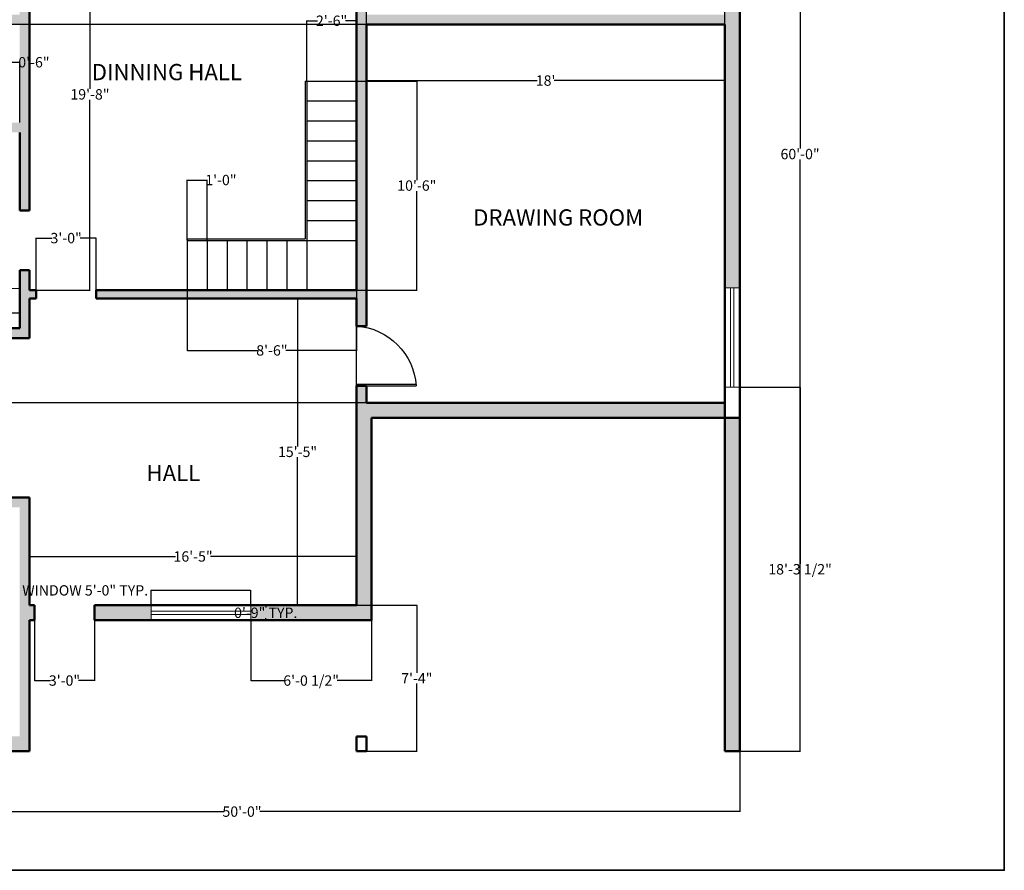
# Model space of a CAD drawing. Units: inches. Extents: x -335 to 1312, y -66 to 821.
# Tile 3 of 4: x 719 to 1312, y -66 to 446. Entities that reach past the tile are written whole.
import ezdxf

# ---------------------------------------------------------------- set-up
doc = ezdxf.new("R2010")
doc.units = ezdxf.units.IN
doc.header["$MEASUREMENT"] = 0
for name, color, linetype, lineweight in [('A-ANNO-DIMS', 2, 'Continuous', 18), ('A-ANNO-TTLB', 7, 'Continuous', 35), ('A-AREA-IDEN', 7, 'Continuous', 25), ('A-COLS', 7, 'Continuous', 50), ('A-DOOR', 34, 'Continuous', 25), ('A-FLOR-FIXT', 8, 'Continuous', 18), ('A-FLOR-STRS', 7, 'Continuous', 25), ('A-GLAZ', 34, 'Continuous', 18), ('A-WALL', 7, 'Continuous', 50), ('A-WALL-PATT', 252, 'Continuous', 13)]:
    doc.layers.add(name, color=color, linetype=linetype, lineweight=lineweight)
doc.styles.get("Standard").update_dxf_attribs({"font": 'arial.ttf'})
doc.dimstyles.get("Standard").update_dxf_attribs({"dimtxt": 6.25, "dimasz": 0.18, "dimexe": 0.18, "dimexo": 0.0625, "dimgap": 0.09, "dimtad": 0, "dimtih": 1, "dimtoh": 1, "dimdec": 0, "dimzin": 0, "dimdsep": 46, "dimlunit": 3, "dimtxsty": 'Standard', "dimcen": 0.09, "dimadec": 0, "dimazin": 0, "dimtfac": 1, "dimtdec": 0, "dimtofl": 0, "dimtmove": 0, "dimatfit": 3, "dimfxl": 1, "dimtolj": 1, "dimtzin": 0, "dimarcsym": 0})

# ---------------------------------------------------------------- blocks, each defined once
blk = doc.blocks.new('*D6')
at = {"layer": 'A-ANNO-DIMS', "color": 0, "lineweight": -2, "transparency": 16777216}
for p, q in [((561.55, 260.47), (561.55, 269.75)), ((561.73, 269.57), (629.52, 269.57)), ((718.37, 269.57), (650.58, 269.57)), ((718.55, 260.47), (718.55, 269.75))]:
    blk.add_line(p, q, dxfattribs=at)
at = {"layer": 'A-ANNO-DIMS', "color": 0, "transparency": 16777216}
for points in [[(561.73, 269.6), (561.73, 269.54), (561.55, 269.57)], [(718.37, 269.6), (718.37, 269.54), (718.55, 269.57)]]:
    blk.add_solid(points, dxfattribs=at)
at = {"layer": 'Defpoints', "color": 0, "transparency": 16777216}
for p in [(561.55, 269.57), (561.55, 260.41), (718.55, 260.41)]:
    blk.add_point(p, dxfattribs=at)
at = {"layer": 'A-ANNO-DIMS', "color": 0, "transparency": 16777216, "insert": (640.05, 269.57), "char_height": 6.25, "attachment_point": 5}
blk.add_mtext('\\A1;13\'-1"', dxfattribs=at)
blk = doc.blocks.new('*D15')
at = {"layer": 'A-ANNO-DIMS', "color": 0, "lineweight": -2, "transparency": 16777216}
for p, q in [((921.49, 278.41), (885.84, 278.41)), ((886.02, 278.23), (886.02, 189.19)), ((886.02, 93.59), (886.02, 182.63)), ((921.49, 93.41), (885.84, 93.41))]:
    blk.add_line(p, q, dxfattribs=at)
at = {"layer": 'A-ANNO-DIMS', "color": 0, "transparency": 16777216}
for points in [[(885.99, 278.23), (886.05, 278.23), (886.02, 278.41)], [(885.99, 93.59), (886.05, 93.59), (886.02, 93.41)]]:
    blk.add_solid(points, dxfattribs=at)
at = {"layer": 'Defpoints', "color": 0, "transparency": 16777216}
for p in [(886.02, 278.41), (921.55, 278.41), (921.55, 93.41)]:
    blk.add_point(p, dxfattribs=at)
at = {"layer": 'A-ANNO-DIMS', "color": 0, "transparency": 16777216, "insert": (886.02, 185.91), "char_height": 6.25, "attachment_point": 5}
blk.add_mtext('\\A1;15\'-5"', dxfattribs=at)
blk = doc.blocks.new('*D16')
at = {"layer": 'A-ANNO-DIMS', "color": 0, "lineweight": -2, "transparency": 16777216}
for p, q in [((724.55, 93.47), (724.55, 123.03)), ((724.73, 122.85), (812.52, 122.85)), ((921.37, 122.85), (833.58, 122.85)), ((921.55, 93.47), (921.55, 123.03))]:
    blk.add_line(p, q, dxfattribs=at)
at = {"layer": 'A-ANNO-DIMS', "color": 0, "transparency": 16777216}
for points in [[(724.73, 122.88), (724.73, 122.82), (724.55, 122.85)], [(921.37, 122.88), (921.37, 122.82), (921.55, 122.85)]]:
    blk.add_solid(points, dxfattribs=at)
at = {"layer": 'Defpoints', "color": 0, "transparency": 16777216}
for p in [(921.55, 122.85), (724.55, 93.41), (921.55, 93.41)]:
    blk.add_point(p, dxfattribs=at)
at = {"layer": 'A-ANNO-DIMS', "color": 0, "transparency": 16777216, "insert": (823.05, 122.85), "char_height": 6.25, "attachment_point": 5}
blk.add_mtext('\\A1;16\'-5"', dxfattribs=at)
blk = doc.blocks.new('*D17')
at = {"layer": 'A-ANNO-DIMS', "color": 0, "lineweight": -2, "transparency": 16777216}
for p, q in [((927.55, 443.35), (927.55, 409.54)), ((1143.55, 443.35), (1143.55, 409.54)), ((927.73, 409.72), (1030.45, 409.72)), ((1143.37, 409.72), (1040.65, 409.72))]:
    blk.add_line(p, q, dxfattribs=at)
at = {"layer": 'A-ANNO-DIMS', "color": 0, "transparency": 16777216}
for points in [[(927.73, 409.75), (927.73, 409.69), (927.55, 409.72)], [(1143.37, 409.75), (1143.37, 409.69), (1143.55, 409.72)]]:
    blk.add_solid(points, dxfattribs=at)
at = {"layer": 'Defpoints', "color": 0, "transparency": 16777216}
for p in [(927.55, 443.41), (1143.55, 443.41), (927.55, 409.72)]:
    blk.add_point(p, dxfattribs=at)
at = {"layer": 'A-ANNO-DIMS', "color": 0, "transparency": 16777216, "insert": (1035.55, 409.72), "char_height": 6.25, "attachment_point": 5}
blk.add_mtext("\\A1;18'", dxfattribs=at)
blk = doc.blocks.new('*D18')
at = {"layer": 'A-ANNO-DIMS', "color": 0, "lineweight": -2, "transparency": 16777216}
for p, q in [((927.55, 443.47), (927.55, 454.59)), ((927.73, 454.41), (1030.45, 454.41)), ((1143.37, 454.41), (1040.65, 454.41)), ((1143.55, 443.47), (1143.55, 454.59))]:
    blk.add_line(p, q, dxfattribs=at)
at = {"layer": 'A-ANNO-DIMS', "color": 0, "transparency": 16777216}
for points in [[(927.73, 454.44), (927.73, 454.38), (927.55, 454.41)], [(1143.37, 454.44), (1143.37, 454.38), (1143.55, 454.41)]]:
    blk.add_solid(points, dxfattribs=at)
at = {"layer": 'Defpoints', "color": 0, "transparency": 16777216}
for p in [(927.55, 454.41), (927.55, 443.41), (1143.55, 443.41)]:
    blk.add_point(p, dxfattribs=at)
at = {"layer": 'A-ANNO-DIMS', "color": 0, "transparency": 16777216, "insert": (1035.55, 454.41), "char_height": 6.25, "attachment_point": 5}
blk.add_mtext("\\A1;18'", dxfattribs=at)
blk = doc.blocks.new('WIN-60IN')
for p, q in [((9, 60), (0, 60)), ((0, 60), (0, 0)), ((3.5, 60), (3.5, 0)), ((5.5, 60), (5.5, 0)), ((9, 0), (9, 60)), ((0, 0), (9, 0))]:
    blk.add_line(p, q)
blk = doc.blocks.new('DOOR-SWING-36IN')
for p, q in [((0, 0), (0, 35.94)), ((1, 0), (1, 35.86)), ((0, 0), (36, 0))]:
    blk.add_line(p, q)
blk.add_arc((-2.68, -2.74), 38.78, 4.05456, 86.03519)
blk = doc.blocks.new('*D29')
at = {"layer": 'A-ANNO-DIMS', "color": 0, "lineweight": -2, "transparency": 16777216}
for p, q in [((797.84, 102.41), (797.66, 102.41)), ((797.84, 93.47), (797.84, 102.59)), ((857.66, 102.41), (798.02, 102.41)), ((857.84, 93.47), (857.84, 102.59))]:
    blk.add_line(p, q, dxfattribs=at)
at = {"layer": 'A-ANNO-DIMS', "color": 0, "transparency": 16777216}
for points in [[(798.02, 102.44), (798.02, 102.38), (797.84, 102.41)], [(857.66, 102.44), (857.66, 102.38), (857.84, 102.41)]]:
    blk.add_solid(points, dxfattribs=at)
at = {"layer": 'Defpoints', "color": 0, "transparency": 16777216}
for p in [(797.84, 102.41), (797.84, 93.41), (857.84, 93.41)]:
    blk.add_point(p, dxfattribs=at)
at = {"layer": 'A-ANNO-DIMS', "color": 0, "transparency": 16777216, "insert": (758.03, 102.41), "char_height": 6.25, "attachment_point": 5}
blk.add_mtext('\\A1;WINDOW 5\'-0" TYP.', dxfattribs=at)
blk = doc.blocks.new('*D30')
at = {"layer": 'A-ANNO-DIMS', "color": 0, "lineweight": -2, "transparency": 16777216}
for p, q in [((857.91, 93.41), (867.02, 93.41)), ((866.84, 93.23), (866.84, 92.19)), ((857.91, 84.41), (867.02, 84.41)), ((866.84, 84.59), (866.84, 85.63))]:
    blk.add_line(p, q, dxfattribs=at)
at = {"layer": 'A-ANNO-DIMS', "color": 0, "transparency": 16777216}
for points in [[(866.81, 93.23), (866.87, 93.23), (866.84, 93.41)], [(866.81, 84.59), (866.87, 84.59), (866.84, 84.41)]]:
    blk.add_solid(points, dxfattribs=at)
at = {"layer": 'Defpoints', "color": 0, "transparency": 16777216}
for p in [(857.84, 93.41), (866.84, 93.41), (857.84, 84.41)]:
    blk.add_point(p, dxfattribs=at)
at = {"layer": 'A-ANNO-DIMS', "color": 0, "transparency": 16777216, "insert": (866.84, 88.91), "char_height": 6.25, "attachment_point": 5}
blk.add_mtext('\\A1;0\'-9" TYP.', dxfattribs=at)
blk = doc.blocks.new('*D31')
at = {"layer": 'A-ANNO-DIMS', "color": 0, "lineweight": -2, "transparency": 16777216}
for p, q in [((552.55, 5.35), (552.55, -31.12)), ((1152.55, 5.35), (1152.55, -31.12)), ((552.73, -30.94), (841.73, -30.94)), ((1152.37, -30.94), (863.38, -30.94))]:
    blk.add_line(p, q, dxfattribs=at)
at = {"layer": 'A-ANNO-DIMS', "color": 0, "transparency": 16777216}
for points in [[(552.73, -30.91), (552.73, -30.97), (552.55, -30.94)], [(1152.37, -30.91), (1152.37, -30.97), (1152.55, -30.94)]]:
    blk.add_solid(points, dxfattribs=at)
at = {"layer": 'Defpoints', "color": 0, "transparency": 16777216}
for p in [(552.55, 5.41), (1152.55, 5.41), (1152.55, -30.94)]:
    blk.add_point(p, dxfattribs=at)
at = {"layer": 'A-ANNO-DIMS', "color": 0, "transparency": 16777216, "insert": (852.55, -30.94), "char_height": 6.25, "attachment_point": 5}
blk.add_mtext('\\A1;50\'-0"', dxfattribs=at)
blk = doc.blocks.new('*D33')
at = {"layer": 'A-ANNO-DIMS', "color": 0, "lineweight": -2, "transparency": 16777216}
for p, q in [((1143.49, 443.41), (516.02, 443.41)), ((516.2, 443.23), (516.2, 332.69)), ((516.2, 215.59), (516.2, 326.13)), ((1143.49, 215.41), (516.02, 215.41))]:
    blk.add_line(p, q, dxfattribs=at)
at = {"layer": 'A-ANNO-DIMS', "color": 0, "transparency": 16777216}
for points in [[(516.17, 443.23), (516.23, 443.23), (516.2, 443.41)], [(516.17, 215.59), (516.23, 215.59), (516.2, 215.41)]]:
    blk.add_solid(points, dxfattribs=at)
at = {"layer": 'Defpoints', "color": 0, "transparency": 16777216}
for p in [(516.2, 443.41), (1143.55, 443.41), (1143.55, 215.41)]:
    blk.add_point(p, dxfattribs=at)
at = {"layer": 'A-ANNO-DIMS', "color": 0, "transparency": 16777216, "insert": (516.2, 329.41), "char_height": 6.25, "attachment_point": 5}
blk.add_mtext('\\A1;19\'-0"', dxfattribs=at)
blk = doc.blocks.new('*D35')
at = {"layer": 'A-ANNO-DIMS', "color": 0, "lineweight": -2, "transparency": 16777216}
for p, q in [((921.613882, 93.408813), (958.081382, 93.408813)), ((957.901382, 93.228813), (957.901382, 52.623813)), ((957.901382, 5.588813), (957.901382, 46.193813)), ((921.613882, 5.408813), (958.081382, 5.408813))]:
    blk.add_line(p, q, dxfattribs=at)
at = {"layer": 'A-ANNO-DIMS', "color": 0, "transparency": 16777216}
for points in [[(957.871382, 93.228813), (957.931382, 93.228813), (957.901382, 93.408813)], [(957.871382, 5.588813), (957.931382, 5.588813), (957.901382, 5.408813)]]:
    blk.add_solid(points, dxfattribs=at)
at = {"layer": 'Defpoints', "color": 0, "transparency": 16777216}
for p in [(921.551382, 93.408813), (921.551382, 5.408813), (957.901382, 5.408813)]:
    blk.add_point(p, dxfattribs=at)
at = {"layer": 'A-ANNO-DIMS', "color": 0, "transparency": 16777216, "insert": (957.901382, 49.408813), "char_height": 6.25, "attachment_point": 5}
blk.add_mtext('\\A1;7\'-4"', dxfattribs=at)
blk = doc.blocks.new('*D39')
at = {"layer": 'A-ANNO-DIMS', "color": 0, "lineweight": -2, "transparency": 16777216}
for p, q in [((1152.61, 224.87), (1189.08, 224.87)), ((1188.9, 224.69), (1188.9, 118.46)), ((1188.9, 5.59), (1188.9, 111.82)), ((1152.61, 5.41), (1189.08, 5.41))]:
    blk.add_line(p, q, dxfattribs=at)
at = {"layer": 'A-ANNO-DIMS', "color": 0, "transparency": 16777216}
for points in [[(1188.87, 224.69), (1188.93, 224.69), (1188.9, 224.87)], [(1188.87, 5.59), (1188.93, 5.59), (1188.9, 5.41)]]:
    blk.add_solid(points, dxfattribs=at)
at = {"layer": 'Defpoints', "color": 0, "transparency": 16777216}
for p in [(1152.55, 224.87), (1152.55, 5.41), (1188.9, 5.41)]:
    blk.add_point(p, dxfattribs=at)
at = {"layer": 'A-ANNO-DIMS', "color": 0, "transparency": 16777216, "insert": (1188.9, 115.14), "char_height": 6.25, "attachment_point": 5}
blk.add_mtext('\\A1;18\'-3 1/2"', dxfattribs=at)
blk = doc.blocks.new('*D41')
at = {"layer": 'A-ANNO-DIMS', "color": 0, "lineweight": -2, "transparency": 16777216}
for p, q in [((857.84, 84.35), (857.84, 47.88)), ((930.55, 84.35), (930.55, 47.88)), ((858.02, 48.06), (878.5, 48.06)), ((930.37, 48.06), (909.89, 48.06))]:
    blk.add_line(p, q, dxfattribs=at)
at = {"layer": 'A-ANNO-DIMS', "color": 0, "transparency": 16777216}
for points in [[(858.02, 48.09), (858.02, 48.03), (857.84, 48.06)], [(930.37, 48.09), (930.37, 48.03), (930.55, 48.06)]]:
    blk.add_solid(points, dxfattribs=at)
at = {"layer": 'Defpoints', "color": 0, "transparency": 16777216}
for p in [(857.84, 84.41), (930.55, 84.41), (857.84, 48.06)]:
    blk.add_point(p, dxfattribs=at)
at = {"layer": 'A-ANNO-DIMS', "color": 0, "transparency": 16777216, "insert": (894.2, 48.06), "char_height": 6.25, "attachment_point": 5}
blk.add_mtext('\\A1;6\'-0 1/2"', dxfattribs=at)
blk = doc.blocks.new('*D42')
at = {"layer": 'A-ANNO-DIMS', "color": 0, "lineweight": -2, "transparency": 16777216}
for p, q in [((1152.61, 725.41), (1189.08, 725.41)), ((1188.9, 725.23), (1188.9, 368.69)), ((1188.9, 5.59), (1188.9, 362.13)), ((1152.61, 5.41), (1189.08, 5.41))]:
    blk.add_line(p, q, dxfattribs=at)
at = {"layer": 'A-ANNO-DIMS', "color": 0, "transparency": 16777216}
for points in [[(1188.87, 725.23), (1188.93, 725.23), (1188.9, 725.41)], [(1188.87, 5.59), (1188.93, 5.59), (1188.9, 5.41)]]:
    blk.add_solid(points, dxfattribs=at)
at = {"layer": 'Defpoints', "color": 0, "transparency": 16777216}
for p in [(1152.55, 725.41), (1188.9, 725.41), (1152.55, 5.41)]:
    blk.add_point(p, dxfattribs=at)
at = {"layer": 'A-ANNO-DIMS', "color": 0, "transparency": 16777216, "insert": (1188.9, 365.41), "char_height": 6.25, "attachment_point": 5}
blk.add_mtext('\\A1;60\'-0"', dxfattribs=at)
blk = doc.blocks.new('*D43')
at = {"layer": 'A-ANNO-DIMS', "color": 0, "lineweight": -2, "transparency": 16777216}
for p, q in [((819.55, 283.35), (819.55, 246.88)), ((921.55, 283.35), (921.55, 246.88)), ((819.73, 247.06), (862.15, 247.06)), ((921.37, 247.06), (878.95, 247.06))]:
    blk.add_line(p, q, dxfattribs=at)
at = {"layer": 'A-ANNO-DIMS', "color": 0, "transparency": 16777216}
for points in [[(819.73, 247.09), (819.73, 247.03), (819.55, 247.06)], [(921.37, 247.09), (921.37, 247.03), (921.55, 247.06)]]:
    blk.add_solid(points, dxfattribs=at)
at = {"layer": 'Defpoints', "color": 0, "transparency": 16777216}
for p in [(819.55, 283.41), (921.55, 283.41), (819.55, 247.06)]:
    blk.add_point(p, dxfattribs=at)
at = {"layer": 'A-ANNO-DIMS', "color": 0, "transparency": 16777216, "insert": (870.55, 247.06), "char_height": 6.25, "attachment_point": 5}
blk.add_mtext('\\A1;8\'-6"', dxfattribs=at)
blk = doc.blocks.new('*D44')
at = {"layer": 'A-ANNO-DIMS', "color": 0, "lineweight": -2, "transparency": 16777216}
for p, q in [((921.61, 409.41), (958.08, 409.41)), ((957.9, 409.23), (957.9, 349.69)), ((957.9, 283.59), (957.9, 343.13)), ((921.61, 283.41), (958.08, 283.41))]:
    blk.add_line(p, q, dxfattribs=at)
at = {"layer": 'A-ANNO-DIMS', "color": 0, "transparency": 16777216}
for points in [[(957.87, 409.23), (957.93, 409.23), (957.9, 409.41)], [(957.87, 283.59), (957.93, 283.59), (957.9, 283.41)]]:
    blk.add_solid(points, dxfattribs=at)
at = {"layer": 'Defpoints', "color": 0, "transparency": 16777216}
for p in [(921.55, 409.41), (921.55, 283.41), (957.9, 283.41)]:
    blk.add_point(p, dxfattribs=at)
at = {"layer": 'A-ANNO-DIMS', "color": 0, "transparency": 16777216, "insert": (957.9, 346.41), "char_height": 6.25, "attachment_point": 5}
blk.add_mtext('\\A1;10\'-6"', dxfattribs=at)
blk = doc.blocks.new('*D45')
at = {"layer": 'A-ANNO-DIMS', "color": 0, "lineweight": -2, "transparency": 16777216}
for p, q in [((891.55, 409.47), (891.55, 445.94)), ((891.73, 445.76), (898.1, 445.76)), ((921.37, 445.76), (915, 445.76)), ((921.55, 409.47), (921.55, 445.94))]:
    blk.add_line(p, q, dxfattribs=at)
at = {"layer": 'A-ANNO-DIMS', "color": 0, "transparency": 16777216}
for points in [[(891.73, 445.79), (891.73, 445.73), (891.55, 445.76)], [(921.37, 445.79), (921.37, 445.73), (921.55, 445.76)]]:
    blk.add_solid(points, dxfattribs=at)
at = {"layer": 'Defpoints', "color": 0, "transparency": 16777216}
for p in [(921.55, 445.76), (891.55, 409.41), (921.55, 409.41)]:
    blk.add_point(p, dxfattribs=at)
at = {"layer": 'A-ANNO-DIMS', "color": 0, "transparency": 16777216, "insert": (906.55, 445.76), "char_height": 6.25, "attachment_point": 5}
blk.add_mtext('\\A1;2\'-6"', dxfattribs=at)
blk = doc.blocks.new('*D46')
at = {"layer": 'A-ANNO-DIMS', "color": 0, "lineweight": -2, "transparency": 16777216}
for p, q in [((819.55, 313.47), (819.55, 349.94)), ((819.73, 349.76), (831.37, 349.76)), ((831.55, 313.47), (831.55, 349.94)), ((831.55, 349.76), (831.73, 349.76))]:
    blk.add_line(p, q, dxfattribs=at)
at = {"layer": 'A-ANNO-DIMS', "color": 0, "transparency": 16777216}
for points in [[(819.73, 349.79), (819.73, 349.73), (819.55, 349.76)], [(831.37, 349.79), (831.37, 349.73), (831.55, 349.76)]]:
    blk.add_solid(points, dxfattribs=at)
at = {"layer": 'Defpoints', "color": 0, "transparency": 16777216}
for p in [(831.55, 349.76), (819.55, 313.41), (831.55, 313.41)]:
    blk.add_point(p, dxfattribs=at)
at = {"layer": 'A-ANNO-DIMS', "color": 0, "transparency": 16777216, "insert": (839.83, 349.76), "char_height": 6.25, "attachment_point": 5}
blk.add_mtext('\\A1;1\'-0"', dxfattribs=at)
blk = doc.blocks.new('*D47')
at = {"layer": 'A-ANNO-DIMS', "color": 0, "lineweight": -2, "transparency": 16777216}
for p, q in [((724.61, 519.41), (761.08, 519.41)), ((760.9, 519.23), (760.9, 404.69)), ((760.9, 283.59), (760.9, 398.13)), ((724.61, 283.41), (761.08, 283.41))]:
    blk.add_line(p, q, dxfattribs=at)
at = {"layer": 'A-ANNO-DIMS', "color": 0, "transparency": 16777216}
for points in [[(760.87, 519.23), (760.93, 519.23), (760.9, 519.41)], [(760.87, 283.59), (760.93, 283.59), (760.9, 283.41)]]:
    blk.add_solid(points, dxfattribs=at)
at = {"layer": 'Defpoints', "color": 0, "transparency": 16777216}
for p in [(724.55, 519.41), (724.55, 283.41), (760.9, 283.41)]:
    blk.add_point(p, dxfattribs=at)
at = {"layer": 'A-ANNO-DIMS', "color": 0, "transparency": 16777216, "insert": (760.9, 401.41), "char_height": 6.25, "attachment_point": 5}
blk.add_mtext('\\A1;19\'-8"', dxfattribs=at)
blk = doc.blocks.new('*D57')
at = {"layer": 'A-ANNO-DIMS', "color": 0, "lineweight": -2, "transparency": 16777216}
for p, q in [((728.55, 278.47), (728.55, 314.94)), ((728.73, 314.76), (738.16, 314.76)), ((764.37, 314.76), (754.95, 314.76)), ((764.55, 278.47), (764.55, 314.94))]:
    blk.add_line(p, q, dxfattribs=at)
at = {"layer": 'A-ANNO-DIMS', "color": 0, "transparency": 16777216}
for points in [[(728.73, 314.79), (728.73, 314.73), (728.55, 314.76)], [(764.37, 314.79), (764.37, 314.73), (764.55, 314.76)]]:
    blk.add_solid(points, dxfattribs=at)
at = {"layer": 'Defpoints', "color": 0, "transparency": 16777216}
for p in [(764.55, 314.76), (728.55, 278.41), (764.55, 278.41)]:
    blk.add_point(p, dxfattribs=at)
at = {"layer": 'A-ANNO-DIMS', "color": 0, "transparency": 16777216, "insert": (746.55, 314.76), "char_height": 6.25, "attachment_point": 5}
blk.add_mtext('\\A1;3\'-0"', dxfattribs=at)
blk = doc.blocks.new('*D58')
at = {"layer": 'A-ANNO-DIMS', "color": 0, "lineweight": -2, "transparency": 16777216}
for p, q in [((727.55, 84.35), (727.55, 47.88)), ((763.55, 84.35), (763.55, 47.88)), ((727.73, 48.06), (737.16, 48.06)), ((763.37, 48.06), (753.95, 48.06))]:
    blk.add_line(p, q, dxfattribs=at)
at = {"layer": 'A-ANNO-DIMS', "color": 0, "transparency": 16777216}
for points in [[(727.73, 48.09), (727.73, 48.03), (727.55, 48.06)], [(763.37, 48.09), (763.37, 48.03), (763.55, 48.06)]]:
    blk.add_solid(points, dxfattribs=at)
at = {"layer": 'Defpoints', "color": 0, "transparency": 16777216}
for p in [(727.55, 84.41), (763.55, 84.41), (727.55, 48.06)]:
    blk.add_point(p, dxfattribs=at)
at = {"layer": 'A-ANNO-DIMS', "color": 0, "transparency": 16777216, "insert": (745.55, 48.06), "char_height": 6.25, "attachment_point": 5}
blk.add_mtext('\\A1;3\'-0"', dxfattribs=at)
blk = doc.blocks.new('*D61')
at = {"layer": 'A-ANNO-DIMS', "color": 0, "lineweight": -2, "transparency": 16777216}
for p, q in [((712.55, 384.47), (712.55, 420.94)), ((712.73, 420.76), (718.37, 420.76)), ((718.55, 384.47), (718.55, 420.94)), ((718.55, 420.76), (718.73, 420.76))]:
    blk.add_line(p, q, dxfattribs=at)
at = {"layer": 'A-ANNO-DIMS', "color": 0, "transparency": 16777216}
for points in [[(712.73, 420.79), (712.73, 420.73), (712.55, 420.76)], [(718.37, 420.79), (718.37, 420.73), (718.55, 420.76)]]:
    blk.add_solid(points, dxfattribs=at)
at = {"layer": 'Defpoints', "color": 0, "transparency": 16777216}
for p in [(718.55, 420.76), (712.55, 384.41), (718.55, 384.41)]:
    blk.add_point(p, dxfattribs=at)
at = {"layer": 'A-ANNO-DIMS', "color": 0, "transparency": 16777216, "insert": (727.13, 420.76), "char_height": 6.25, "attachment_point": 5}
blk.add_mtext('\\A1;0\'-6"', dxfattribs=at)

msp = doc.modelspace()

# ---------------------------------------------------------------- hatches: boundary and pattern name
at = {"layer": 'A-WALL-PATT'}
h = msp.add_hatch(color=256, dxfattribs=at)
h.dxf.hatch_style = 1
h.paths.add_polyline_path([(561.55, 92.41), (552.55, 92.41), (552.55, 5.41), (724.55, 5.41), (724.55, 84.41), (727.55, 84.41), (727.55, 93.41), (724.55, 93.41), (724.55, 158.41), (712.55, 158.41), (712.55, 152.41), (718.55, 152.41), (718.55, 14.41), (561.55, 14.41)])
h.paths.add_polyline_path([(561.55, 254.41), (657.55, 254.41), (657.55, 200.41), (663.55, 200.41), (663.55, 254.41), (724.55, 254.41), (724.55, 278.41), (728.55, 278.41), (728.55, 283.41), (724.55, 283.41), (724.55, 295.41), (718.55, 295.41), (718.55, 260.41), (561.55, 260.41), (561.55, 318.41), (552.55, 318.41), (552.55, 152.41), (561.55, 152.41), (676.55, 152.41), (676.55, 158.41), (663.55, 158.41), (663.55, 164.41), (657.55, 164.41), (657.55, 158.41), (561.55, 158.41)])
h.paths.add_polyline_path([(561.55, 443.41), (634.55, 443.41), (634.55, 384.41), (634.55, 378.41), (676.55, 378.41), (676.55, 384.41), (640.55, 384.41), (640.55, 443.41), (718.55, 443.41), (718.55, 384.41), (712.55, 384.41), (712.55, 378.41), (718.55, 378.41), (718.55, 331.41), (724.55, 331.41), (724.55, 454.41), (718.55, 454.41), (718.55, 449.41), (561.55, 449.41), (561.55, 535.84), (552.55, 535.84), (552.55, 378.41), (561.55, 378.41), (598.55, 378.41), (598.55, 384.41), (561.55, 384.41)])
h.paths.add_polyline_path([(724.55, 725.41), (552.55, 725.41), (552.55, 595.84), (561.55, 595.84), (561.55, 626.41), (566.55, 626.41), (566.55, 632.41), (561.55, 632.41), (561.55, 716.41), (718.55, 716.41), (718.55, 632.41), (602.55, 632.41), (602.55, 626.41), (718.55, 626.41), (718.55, 490.41), (724.55, 490.41), (724.55, 519.41), (772.54, 519.41), (772.56, 525.41), (724.55, 525.41)])
h.paths.add_polyline_path([(927.55, 716.41), (1143.55, 716.41), (1143.55, 632.41), (1139.31, 632.41), (1139.31, 626.41), (1143.55, 626.41), (1143.55, 598.07), (1152.55, 598.07), (1152.55, 725.41), (921.55, 725.41), (921.55, 598.41), (921.55, 525.41), (904.55, 525.41), (904.55, 519.41), (921.55, 519.41), (921.55, 490.41), (927.55, 490.41), (927.55, 626.41), (1103.31, 626.41), (1103.31, 632.41), (927.55, 632.41)])
h.paths.add_polyline_path([(1152.55, 538.07), (1143.55, 538.07), (1143.55, 449.41), (927.55, 449.41), (927.55, 454.41), (921.55, 454.41), (921.55, 283.41), (764.57, 283.41), (764.55, 278.41), (921.55, 278.41), (921.55, 261.75), (927.55, 261.75), (927.55, 443.41), (1143.55, 443.41), (1143.55, 284.87), (1152.55, 284.87)])
h.paths.add_polyline_path([(930.55, 206.41), (1143.55, 206.41), (1143.55, 215.41), (927.55, 215.41), (927.55, 225.75), (921.55, 225.75), (921.55, 93.41), (857.84, 93.41), (857.84, 84.41), (930.55, 84.41)])
h.paths.add_polyline_path([(1152.55, 206.41), (1143.55, 206.41), (1143.55, 5.41), (1152.55, 5.41)])
h.paths.add_polyline_path([(797.84, 93.41), (763.55, 93.41), (763.55, 84.41), (797.84, 84.41)])

# ---------------------------------------------------------------- linework, layer by layer
at = {"layer": 'A-ANNO-TTLB'}
msp.add_lwpolyline([(405.31, 821.01), (1312, 821.01), (1312, -66.33), (405.31, -66.33)], close=True, dxfattribs=at)
at = {"layer": 'A-COLS'}
for p, q in [((921.55, 14.41), (927.55, 14.41)), ((921.55, 14.41), (921.55, 5.41)), ((927.55, 14.41), (927.55, 5.41)), ((921.55, 5.41), (927.55, 5.41))]:
    msp.add_line(p, q, dxfattribs=at)
at = {"layer": 'A-FLOR-FIXT'}
msp.add_line((718.55, 284.41), (585.55, 284.41), dxfattribs=at)
at = {"layer": 'A-FLOR-STRS'}
for p, q in [((890.55, 409.41), (921.55, 409.41)), ((890.55, 409.41), (890.55, 314.41)), ((891.55, 409.41), (891.55, 283.41)), ((891.55, 397.41), (921.55, 397.41)), ((891.55, 385.41), (921.55, 385.41)), ((891.55, 373.41), (921.55, 373.41)), ((891.55, 361.41), (921.55, 361.41)), ((891.55, 349.41), (921.55, 349.41)), ((891.55, 337.41), (921.55, 337.41)), ((891.55, 325.41), (921.55, 325.41)), ((819.55, 314.41), (819.55, 283.41)), ((819.55, 314.41), (890.55, 314.41)), ((819.55, 313.41), (921.55, 313.41)), ((831.55, 313.41), (831.55, 283.41)), ((843.55, 313.41), (843.55, 283.41)), ((855.55, 313.41), (855.55, 283.41)), ((855.55, 313.41), (855.55, 283.41)), ((867.55, 313.41), (867.55, 283.41)), ((879.55, 313.41), (879.55, 283.41))]:
    msp.add_line(p, q, dxfattribs=at)
at = {"layer": 'A-WALL'}
for p, q in [((1152.55, 245.41), (1152.55, 725.41)), ((724.55, 454.41), (724.55, 331.41)), ((921.55, 454.41), (921.55, 283.41)), ((1143.55, 443.41), (927.55, 443.41)), ((927.55, 443.41), (927.55, 261.75)), ((1143.55, 5.41), (1143.55, 443.41)), ((718.55, 378.41), (718.55, 331.41)), ((724.55, 331.41), (718.55, 331.41)), ((724.55, 295.41), (718.55, 295.41)), ((718.55, 295.41), (718.55, 260.41)), ((724.55, 295.41), (724.55, 283.41)), ((724.55, 283.41), (728.55, 283.41)), ((728.55, 283.41), (728.55, 278.41)), ((764.55, 283.41), (921.55, 283.41)), ((764.57, 283.41), (764.55, 278.41)), ((724.55, 278.41), (728.55, 278.41)), ((724.55, 278.41), (724.55, 254.41)), ((764.55, 278.41), (921.55, 278.41)), ((921.55, 278.41), (921.55, 261.75)), ((927.55, 261.75), (921.55, 261.75)), ((718.55, 260.41), (561.55, 260.41)), ((724.55, 254.41), (663.55, 254.41)), ((1152.55, 5.41), (1152.55, 245.41)), ((927.55, 225.75), (921.55, 225.75)), ((921.55, 225.75), (921.55, 93.41)), ((927.55, 225.75), (927.55, 215.41)), ((1143.55, 215.41), (927.55, 215.41)), ((1152.55, 206.41), (930.55, 206.41)), ((930.55, 206.41), (930.55, 84.41)), ((712.55, 158.41), (724.55, 158.41)), ((724.55, 158.41), (724.55, 93.41)), ((724.55, 93.41), (727.55, 93.41)), ((727.55, 84.41), (727.55, 93.41)), ((763.55, 84.41), (763.55, 93.41)), ((763.55, 93.41), (921.55, 93.41)), ((724.55, 84.41), (727.55, 84.41)), ((724.55, 84.41), (724.55, 5.41)), ((763.55, 84.41), (930.55, 84.41)), ((552.55, 5.41), (724.55, 5.41)), ((1143.55, 5.41), (1152.55, 5.41))]:
    msp.add_line(p, q, dxfattribs=at)

# ---------------------------------------------------------------- block references
at = {"layer": 'A-DOOR', "extrusion": (0, 0, -1), "zscale": -1, "rotation": 90.00000000000024}
msp.add_blockref('DOOR-SWING-36IN', (-921.55, 225.75), dxfattribs=at)
at = {"layer": 'A-GLAZ'}
msp.add_blockref('WIN-60IN', (1143.55, 224.87), dxfattribs=at)
at = {"layer": 'A-GLAZ', "rotation": 89.99999999999999}
msp.add_blockref('WIN-60IN', (857.84, 84.41), dxfattribs=at)

# ---------------------------------------------------------------- texts
at = {"layer": 'A-AREA-IDEN'}
for s, height, p in [('DINNING HALL', 9.7886, (761.98, 409.93)), ('DRAWING ROOM', 9.7886, (991.89, 322.31)), ('HALL', 9.789, (795, 168.29))]:
    msp.add_text(s, height=height, dxfattribs=at).set_placement(p)

# ---------------------------------------------------------------- dimensions: what is measured, and where the dimension line sits
at = {"layer": 'A-ANNO-DIMS'}
for base, p1, p2, angle, override, picture, middle in [((1188.9, 725.41), (1152.55, 5.41), (1152.55, 725.41), 90, {"dimdec": 1, "dimlfac": 1, "dimrnd": 0, "dimzin": 1, "dimdsep": 46, "dimlunit": 4, "dimfrac": 2}, '*D42', (1188.9, 365.41)), ((760.9, 283.41), (724.55, 519.41), (724.55, 283.41), 270, {"dimdec": 1, "dimlfac": 1, "dimrnd": 0, "dimzin": 1, "dimdsep": 46, "dimlunit": 4, "dimfrac": 2}, '*D47', (760.9, 401.41)), ((516.2, 443.41), (1143.55, 215.41), (1143.55, 443.41), 90, {"dimdec": 1, "dimlfac": 1, "dimrnd": 0, "dimzin": 1, "dimdsep": 46, "dimlunit": 4, "dimfrac": 2}, '*D33', (516.2, 329.41)), ((957.9, 283.41), (921.55, 409.41), (921.55, 283.41), 270, {"dimdec": 1, "dimlfac": 1, "dimrnd": 0, "dimzin": 1, "dimdsep": 46, "dimlunit": 4, "dimfrac": 2}, '*D44', (957.9, 346.41)), ((819.55, 247.06), (921.55, 283.41), (819.55, 283.41), 180, {"dimdec": 1, "dimlfac": 1, "dimrnd": 0, "dimzin": 1, "dimdsep": 46, "dimlunit": 4, "dimfrac": 2}, '*D43', (870.55, 247.06)), ((886.02, 278.41), (921.55, 93.41), (921.55, 278.41), 90, {"dimclrd": 0, "dimclre": 0, "dimclrt": 0}, '*D15', (886.02, 185.91)), ((1188.9, 5.41), (1152.55, 224.87), (1152.55, 5.41), 270, {"dimdec": 1, "dimlfac": 1, "dimrnd": 0, "dimzin": 1, "dimdsep": 46, "dimlunit": 4, "dimfrac": 2}, '*D39', (1188.9, 115.14)), ((957.9, 5.41), (921.55, 93.41), (921.55, 5.41), 270, {"dimdec": 1, "dimlfac": 1, "dimrnd": 0, "dimzin": 1, "dimdsep": 46, "dimlunit": 4, "dimfrac": 2}, '*D35', (957.9, 49.41)), ((727.55, 48.06), (763.55, 84.41), (727.55, 84.41), 180, {"dimdec": 1, "dimlfac": 1, "dimrnd": 0, "dimzin": 1, "dimdsep": 46, "dimlunit": 4, "dimfrac": 2}, '*D58', (745.55, 48.06)), ((857.84, 48.06), (930.55, 84.41), (857.84, 84.41), 180, {"dimdec": 1, "dimlfac": 1, "dimrnd": 0, "dimzin": 1, "dimdsep": 46, "dimlunit": 4, "dimfrac": 2}, '*D41', (894.2, 48.06))]:
    dim = msp.add_linear_dim(base=base, p1=p1, p2=p2, angle=angle, dimstyle='Standard', override=override, dxfattribs=at)
    dim.commit()
    dim.dimension.update_dxf_attribs({"geometry": picture, "text_midpoint": middle})
for base, p1, p2, override, picture, middle in [((927.55, 454.41), (1143.55, 443.41), (927.55, 443.41), {"dimclrd": 0, "dimclre": 0, "dimclrt": 0}, '*D18', (1035.55, 454.41)), ((921.55, 445.76), (891.55, 409.41), (921.55, 409.41), {"dimdec": 1, "dimlfac": 1, "dimrnd": 0, "dimzin": 1, "dimdsep": 46, "dimlunit": 4, "dimfrac": 2}, '*D45', (906.55, 445.76)), ((927.55, 409.72), (1143.55, 443.41), (927.55, 443.41), {"dimclrd": 0, "dimclre": 0, "dimclrt": 0}, '*D17', (1035.55, 409.72)), ((718.55, 420.76), (712.55, 384.41), (718.55, 384.41), {"dimdec": 1, "dimlfac": 1, "dimrnd": 0, "dimzin": 1, "dimdsep": 46, "dimlunit": 4, "dimfrac": 2}, '*D61', (727.13, 420.76)), ((831.55, 349.76), (819.55, 313.41), (831.55, 313.41), {"dimdec": 1, "dimlfac": 1, "dimrnd": 0, "dimzin": 1, "dimdsep": 46, "dimlunit": 4, "dimfrac": 2}, '*D46', (839.83, 349.76)), ((764.55, 314.76), (728.55, 278.41), (764.55, 278.41), {"dimdec": 1, "dimlfac": 1, "dimrnd": 0, "dimzin": 1, "dimdsep": 46, "dimlunit": 4, "dimfrac": 2}, '*D57', (746.55, 314.76)), ((561.55, 269.57), (718.55, 260.41), (561.55, 260.41), {"dimclrd": 0, "dimclre": 0, "dimclrt": 0}, '*D6', (640.05, 269.57)), ((921.55, 122.85), (724.55, 93.41), (921.55, 93.41), {"dimclrd": 0, "dimclre": 0, "dimclrt": 0}, '*D16', (823.05, 122.85)), ((1152.55, -30.94), (552.55, 5.41), (1152.55, 5.41), {"dimdec": 1, "dimlfac": 1, "dimrnd": 0, "dimzin": 1, "dimdsep": 46, "dimlunit": 4, "dimfrac": 2}, '*D31', (852.55, -30.94))]:
    dim = msp.add_linear_dim(base=base, p1=p1, p2=p2, dimstyle='Standard', override=override, dxfattribs=at)
    dim.commit()
    dim.dimension.update_dxf_attribs({"geometry": picture, "text_midpoint": middle})
for base, p1, p2, angle, text, picture, middle in [((797.84, 102.41), (857.84, 93.41), (797.84, 93.41), 180, 'WINDOW <> TYP.', '*D29', (758.03, 102.41)), ((866.84, 93.41), (857.84, 84.41), (857.84, 93.41), 90, '<> TYP.', '*D30', (866.84, 88.91))]:
    dim = msp.add_linear_dim(base=base, p1=p1, p2=p2, angle=angle, text=text, dimstyle='Standard', override={"dimdec": 1, "dimlfac": 1, "dimrnd": 0, "dimzin": 1, "dimdsep": 46, "dimlunit": 4, "dimfrac": 2}, dxfattribs=at)
    dim.commit()
    dim.dimension.update_dxf_attribs({"geometry": picture, "text_midpoint": middle})

doc.saveas('drawing.dxf')
